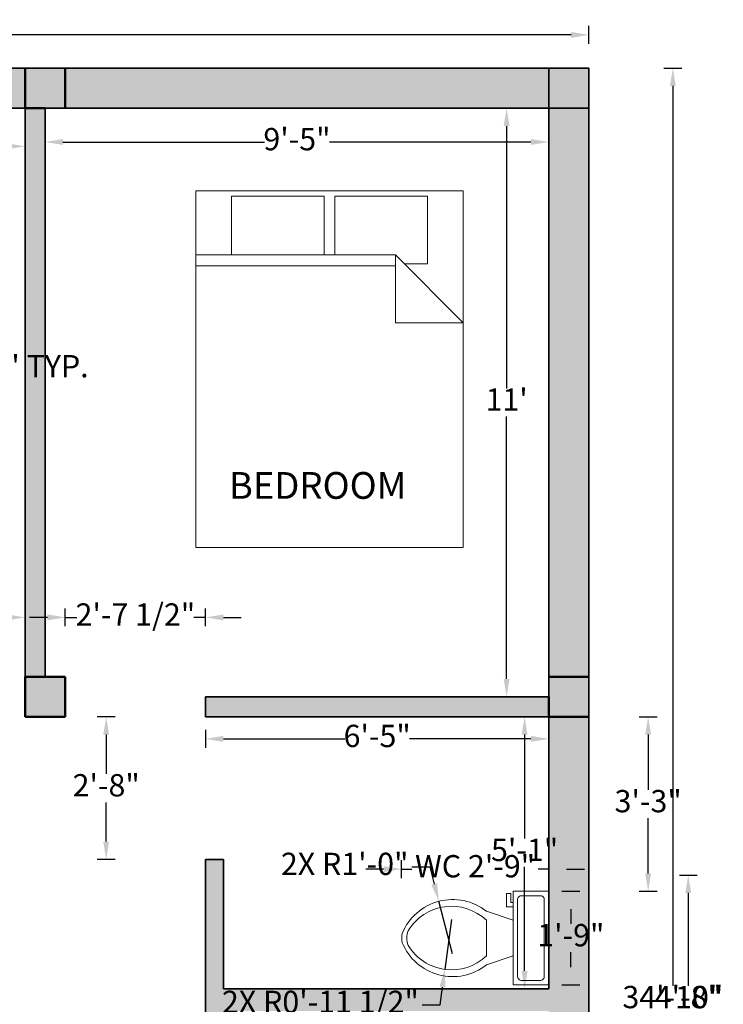
# Model space of a CAD drawing. Units: inches. Extents: x 2244 to 2676, y 593 to 1067.
# Tile 4 of 4: x 2518 to 2676, y 831 to 1052. Entities that reach past the tile are written whole.
import ezdxf

# ---------------------------------------------------------------- set-up
doc = ezdxf.new("R2010")
doc.units = ezdxf.units.IN
for name, color, linetype, lineweight in [('A-ANNO-DIMS', 2, 'Continuous', 18), ('A-AREA-IDEN', 7, 'Continuous', 25), ('A-COLS', 7, 'Continuous', 50), ('A-COLS-PATT', 1, 'Continuous', 13), ('A-FLOR-FIXT', 9, 'Continuous', 18), ('A-FURN', 8, 'Continuous', 18), ('A-WALL', 7, 'Continuous', 35)]:
    doc.layers.add(name, color=color, linetype=linetype, lineweight=lineweight)
doc.layers.add('A-WALL-PATT', color=159, linetype='Continuous', lineweight=13, true_color=0x22346e)
doc.styles.get("Standard").update_dxf_attribs({"font": 'arial.ttf'})
doc.dimstyles.new('ISO-25', dxfattribs={"dimtxt": 5, "dimasz": 4, "dimexe": 2, "dimexo": 2, "dimtad": 0, "dimtih": 1, "dimtoh": 1, "dimlunit": 3, "dimtxsty": 'Standard', "dimcen": 2.5, "dimadec": 0, "dimazin": 0, "dimtfac": 1, "dimtmove": 0, "dimatfit": 3, "dimfxl": 2, "dimfxlon": 1, "dimarcsym": 0})

# ---------------------------------------------------------------- blocks, each defined once
blk = doc.blocks.new('*D6')
at = {"layer": 'A-ANNO-DIMS', "color": 0, "lineweight": -2, "transparency": 16777216}
for p, q in [((2402.7, 1023.38), (2402.7, 1025.38)), ((2519.7, 1023.38), (2519.7, 1025.38)), ((2406.7, 1023.38), (2453.93, 1023.38)), ((2515.7, 1023.38), (2468.47, 1023.38))]:
    blk.add_line(p, q, dxfattribs=at)
at = {"layer": 'A-ANNO-DIMS', "color": 0, "transparency": 16777216}
for points in [[(2406.7, 1024.05), (2406.7, 1022.72), (2402.7, 1023.38)], [(2515.7, 1024.05), (2515.7, 1022.72), (2519.7, 1023.38)]]:
    blk.add_solid(points, dxfattribs=at)
at = {"layer": 'Defpoints', "color": 0, "transparency": 16777216}
for p in [(2402.7, 1023.38), (2402.7, 1022.02), (2519.7, 1022.02)]:
    blk.add_point(p, dxfattribs=at)
at = {"layer": 'A-ANNO-DIMS', "color": 0, "transparency": 16777216, "insert": (2461.2, 1023.38), "char_height": 5, "attachment_point": 5}
blk.add_mtext('9\'-9"', dxfattribs=at)
blk = doc.blocks.new('*D8')
at = {"layer": 'A-ANNO-DIMS', "color": 0, "lineweight": -2, "transparency": 16777216}
for p, q in [((2524.2, 1023.09), (2524.2, 1026.34)), ((2637.2, 1023.09), (2637.2, 1026.34)), ((2528.2, 1024.34), (2573.43, 1024.34)), ((2633.2, 1024.34), (2587.97, 1024.34))]:
    blk.add_line(p, q, dxfattribs=at)
at = {"layer": 'A-ANNO-DIMS', "color": 0, "transparency": 16777216}
for points in [[(2528.2, 1025.01), (2528.2, 1023.68), (2524.2, 1024.34)], [(2633.2, 1025.01), (2633.2, 1023.68), (2637.2, 1024.34)]]:
    blk.add_solid(points, dxfattribs=at)
at = {"layer": 'Defpoints', "color": 0, "transparency": 16777216}
for p in [(2524.2, 1024.34), (2524.2, 1021.09), (2637.2, 1021.09)]:
    blk.add_point(p, dxfattribs=at)
at = {"layer": 'A-ANNO-DIMS', "color": 0, "transparency": 16777216, "insert": (2580.7, 1024.34), "char_height": 5, "attachment_point": 5}
blk.add_mtext('9\'-5"', dxfattribs=at)
blk = doc.blocks.new('*D9')
at = {"layer": 'A-ANNO-DIMS', "color": 0, "lineweight": -2, "transparency": 16777216}
for p, q in [((2626.95, 1031.92), (2629.74, 1031.92)), ((2627.74, 1027.92), (2627.74, 969.06)), ((2627.74, 903.92), (2627.74, 962.79)), ((2626.95, 899.92), (2629.74, 899.92))]:
    blk.add_line(p, q, dxfattribs=at)
at = {"layer": 'A-ANNO-DIMS', "color": 0, "transparency": 16777216}
for points in [[(2627.08, 1027.92), (2628.41, 1027.92), (2627.74, 1031.92)], [(2627.08, 903.92), (2628.41, 903.92), (2627.74, 899.92)]]:
    blk.add_solid(points, dxfattribs=at)
at = {"layer": 'Defpoints', "color": 0, "transparency": 16777216}
for p in [(2624.95, 1031.92), (2624.95, 899.92), (2627.74, 899.92)]:
    blk.add_point(p, dxfattribs=at)
at = {"layer": 'A-ANNO-DIMS', "color": 0, "transparency": 16777216, "insert": (2627.74, 965.92), "char_height": 5, "attachment_point": 5}
blk.add_mtext("11'", dxfattribs=at)
blk = doc.blocks.new('*D11')
at = {"layer": 'A-ANNO-DIMS', "color": 0, "lineweight": -2, "transparency": 16777216}
for p, q in [((2633.78, 895.42), (2629.78, 895.42)), ((2631.78, 891.42), (2631.78, 868.1)), ((2631.78, 838.42), (2631.78, 861.74)), ((2633.78, 834.42), (2629.78, 834.42))]:
    blk.add_line(p, q, dxfattribs=at)
at = {"layer": 'A-ANNO-DIMS', "color": 0, "transparency": 16777216}
for points in [[(2631.11, 891.42), (2632.44, 891.42), (2631.78, 895.42)], [(2631.11, 838.42), (2632.44, 838.42), (2631.78, 834.42)]]:
    blk.add_solid(points, dxfattribs=at)
at = {"layer": 'Defpoints', "color": 0, "transparency": 16777216}
for p in [(2637.2, 895.42), (2631.78, 834.42), (2637.2, 834.42)]:
    blk.add_point(p, dxfattribs=at)
at = {"layer": 'A-ANNO-DIMS', "color": 0, "transparency": 16777216, "insert": (2631.78, 864.92), "char_height": 5, "attachment_point": 5}
blk.add_mtext('5\'-1"', dxfattribs=at)
blk = doc.blocks.new('*D21')
at = {"layer": 'A-ANNO-DIMS', "color": 0, "lineweight": -2, "transparency": 16777216}
for p, q in [((2276.2, 1046.37), (2276.2, 1050.37)), ((2646.2, 1046.37), (2646.2, 1050.37)), ((2280.2, 1048.37), (2450.04, 1048.37)), ((2642.2, 1048.37), (2472.35, 1048.37))]:
    blk.add_line(p, q, dxfattribs=at)
at = {"layer": 'A-ANNO-DIMS', "color": 0, "transparency": 16777216}
for points in [[(2280.2, 1049.03), (2280.2, 1047.7), (2276.2, 1048.37)], [(2642.2, 1049.03), (2642.2, 1047.7), (2646.2, 1048.37)]]:
    blk.add_solid(points, dxfattribs=at)
at = {"layer": 'Defpoints', "color": 0, "transparency": 16777216}
for p in [(2646.2, 1048.37), (2276.2, 1040.92), (2646.2, 1040.92)]:
    blk.add_point(p, dxfattribs=at)
at = {"layer": 'A-ANNO-DIMS', "color": 0, "transparency": 16777216, "insert": (2461.2, 1048.37), "char_height": 5, "attachment_point": 5}
blk.add_mtext('30\'-10"', dxfattribs=at)
blk = doc.blocks.new('*D22')
at = {"layer": 'A-ANNO-DIMS', "color": 0, "lineweight": -2, "transparency": 16777216}
for p, q in [((2663.04, 1040.92), (2667.04, 1040.92)), ((2665.04, 1036.92), (2665.04, 835.1)), ((2665.04, 626.92), (2665.04, 828.74)), ((2663.04, 622.92), (2667.04, 622.92))]:
    blk.add_line(p, q, dxfattribs=at)
at = {"layer": 'A-ANNO-DIMS', "color": 0, "transparency": 16777216}
for points in [[(2664.38, 1036.92), (2665.71, 1036.92), (2665.04, 1040.92)], [(2664.38, 626.92), (2665.71, 626.92), (2665.04, 622.92)]]:
    blk.add_solid(points, dxfattribs=at)
at = {"layer": 'Defpoints', "color": 0, "transparency": 16777216}
for p in [(2646.2, 1040.92), (2646.2, 622.92), (2665.04, 622.92)]:
    blk.add_point(p, dxfattribs=at)
at = {"layer": 'A-ANNO-DIMS', "color": 0, "transparency": 16777216, "insert": (2665.04, 831.92), "char_height": 5, "attachment_point": 5}
blk.add_mtext('34\'-10"', dxfattribs=at)
blk = doc.blocks.new('Bed - Queen')
for p, q in [((0, -80.00003), (0, 0)), ((0, 0), (59.99999, 0)), ((59.99999, 0), (59.99999, -80.00003)), ((7.99999, -1.2), (28.79998, -1.2)), ((7.99999, -14.4), (7.99999, -1.2)), ((28.79998, -1.2), (28.79998, -14.4)), ((31.19999, -1.2), (51.99999, -1.2)), ((31.19999, -14.4), (31.19999, -1.2)), ((51.99999, -1.2), (51.99999, -16.4)), ((0, -14.4), (44.8, -14.4)), ((59.99999, -29.6), (44.8, -14.4)), ((44.8, -14.4), (44.8, -29.6)), ((44.8, -16.8), (0, -16.8)), ((51.99999, -16.4), (46.79936, -16.4)), ((44.8, -29.6), (59.99999, -29.6)), ((59.99999, -80.00003), (0, -80.00003))]:
    blk.add_line(p, q)
blk = doc.blocks.new('Toilet - top')
for p, q in [((9.5, -6), (9.5, -2)), ((-10, -8.5), (-8, -8.5)), ((-10, -9.5), (-10, -8.5)), ((-8, -8.5), (-8, -8)), ((-7, -8), (-7, -9.5)), ((-4, -8), (-6, -14)), ((4, -8), (6, -14)), ((-7, -9.5), (-10, -9.5)), ((4, -14), (-4, -14))]:
    blk.add_line(p, q)
blk.add_lwpolyline([(10.5, -8), (10.5, 0), (-10.5, 0), (-10.5, -8)], close=True)
for points in [[(-9.5, -2), (-9.5, -6)], [(8.5, -1), (-8.5, -1)], [(-8.5, -7), (8.5, -7)]]:
    blk.add_lwpolyline(points)
for centre, radius, start, end in [((-8.62, -1.88), 0.884, 81.8699, 188.1301), ((8.62, -1.88), 0.884, 351.8699, 98.1301), ((-8.62, -6.12), 0.884, 171.8699, 278.1301), ((8.62, -6.12), 0.884, 261.8699, 8.1301), ((3.52, -21.58), 12.17, 141.4691, 247.9714), ((4.2, -21.82), 11.33, 136.3677, 238.9468), ((-3.52, -21.58), 12.17, 292.0284, 38.5307), ((-4.2, -21.82), 11.33, 301.053, 43.6321), ((0, -27.88), 4, 245.7318, 294.2682), ((0, -29), 4, 254.8605, 285.1395)]:
    blk.add_arc(centre, radius, start, end)
blk = doc.blocks.new('*D29')
at = {"layer": 'A-ANNO-DIMS', "color": 0, "lineweight": -2, "transparency": 16777216}
for p, q in [((2560.2, 892.48), (2560.2, 888.48)), ((2637.2, 892.48), (2637.2, 888.48)), ((2564.2, 890.48), (2591.41, 890.48)), ((2633.2, 890.48), (2605.98, 890.48))]:
    blk.add_line(p, q, dxfattribs=at)
at = {"layer": 'A-ANNO-DIMS', "color": 0, "transparency": 16777216}
for points in [[(2564.2, 891.15), (2564.2, 889.81), (2560.2, 890.48)], [(2633.2, 891.15), (2633.2, 889.81), (2637.2, 890.48)]]:
    blk.add_solid(points, dxfattribs=at)
at = {"layer": 'Defpoints', "color": 0, "transparency": 16777216}
for p in [(2560.2, 895.42), (2637.2, 895.42), (2637.2, 890.48)]:
    blk.add_point(p, dxfattribs=at)
at = {"layer": 'A-ANNO-DIMS', "color": 0, "transparency": 16777216, "insert": (2598.7, 890.48), "char_height": 5, "attachment_point": 5}
blk.add_mtext('6\'-5"', dxfattribs=at)
blk = doc.blocks.new('*D30')
at = {"layer": 'A-ANNO-DIMS', "color": 0, "lineweight": -2, "transparency": 16777216}
for p, q in [((2497.1, 1013.41), (2501.1, 1013.41)), ((2499.1, 1009.41), (2499.1, 976.77)), ((2499.1, 937.41), (2499.1, 970.04)), ((2497.1, 933.41), (2501.1, 933.41))]:
    blk.add_line(p, q, dxfattribs=at)
at = {"layer": 'A-ANNO-DIMS', "color": 0, "transparency": 16777216}
for points in [[(2498.44, 1009.41), (2499.77, 1009.41), (2499.1, 1013.41)], [(2498.44, 937.41), (2499.77, 937.41), (2499.1, 933.41)]]:
    blk.add_solid(points, dxfattribs=at)
at = {"layer": 'Defpoints', "color": 0, "transparency": 16777216}
for p in [(2487.1, 1013.41), (2499.1, 1013.41), (2487.1, 933.41)]:
    blk.add_point(p, dxfattribs=at)
at = {"layer": 'A-ANNO-DIMS', "color": 0, "transparency": 16777216, "insert": (2499.1, 973.41), "char_height": 5, "attachment_point": 5}
blk.add_mtext('QUEEN BED 6\'-8" TYP.', dxfattribs=at)
blk = doc.blocks.new('*D34')
at = {"layer": 'A-ANNO-DIMS', "color": 0, "lineweight": -2, "transparency": 16777216}
for p, q in [((2600.15, 861.26), (2596.15, 861.26)), ((2604.15, 859.26), (2604.15, 863.26)), ((2604.15, 861.26), (2606.51, 861.26)), ((2637.2, 861.26), (2634.84, 861.26)), ((2637.2, 859.26), (2637.2, 863.26)), ((2641.2, 861.26), (2645.2, 861.26))]:
    blk.add_line(p, q, dxfattribs=at)
at = {"layer": 'A-ANNO-DIMS', "color": 0, "transparency": 16777216}
for points in [[(2600.15, 861.92), (2600.15, 860.59), (2604.15, 861.26)], [(2641.2, 861.92), (2641.2, 860.59), (2637.2, 861.26)]]:
    blk.add_solid(points, dxfattribs=at)
at = {"layer": 'Defpoints', "color": 0, "transparency": 16777216}
for p in [(2637.2, 861.26), (2604.15, 856.3), (2637.2, 856.3)]:
    blk.add_point(p, dxfattribs=at)
at = {"layer": 'A-ANNO-DIMS', "color": 0, "transparency": 16777216, "insert": (2620.67, 861.26), "char_height": 5, "attachment_point": 5}
blk.add_mtext('WC 2\'-9"', dxfattribs=at)
blk = doc.blocks.new('*D35')
at = {"layer": 'A-ANNO-DIMS', "color": 0, "lineweight": -2, "transparency": 16777216}
for p, q in [((2640.15, 856.3), (2644.15, 856.3)), ((2642.15, 852.3), (2642.15, 848.98)), ((2642.15, 839.3), (2642.15, 842.62)), ((2640.15, 835.3), (2644.15, 835.3))]:
    blk.add_line(p, q, dxfattribs=at)
at = {"layer": 'A-ANNO-DIMS', "color": 0, "transparency": 16777216}
for points in [[(2641.49, 852.3), (2642.82, 852.3), (2642.15, 856.3)], [(2641.49, 839.3), (2642.82, 839.3), (2642.15, 835.3)]]:
    blk.add_solid(points, dxfattribs=at)
at = {"layer": 'Defpoints', "color": 0, "transparency": 16777216}
for p in [(2637.2, 856.3), (2637.2, 835.3), (2642.15, 835.3)]:
    blk.add_point(p, dxfattribs=at)
at = {"layer": 'A-ANNO-DIMS', "color": 0, "transparency": 16777216, "insert": (2642.15, 845.8), "char_height": 5, "attachment_point": 5}
blk.add_mtext('1\'-9"', dxfattribs=at)
blk = doc.blocks.new('*D42')
at = {"layer": 'A-ANNO-DIMS', "color": 0, "lineweight": -2, "transparency": 16777216}
for p, q in [((2666.5, 859.92), (2670.5, 859.92)), ((2668.5, 855.92), (2668.5, 835.1)), ((2668.5, 807.92), (2668.5, 828.74)), ((2666.5, 803.92), (2670.5, 803.92))]:
    blk.add_line(p, q, dxfattribs=at)
at = {"layer": 'A-ANNO-DIMS', "color": 0, "transparency": 16777216}
for points in [[(2667.83, 855.92), (2669.16, 855.92), (2668.5, 859.92)], [(2667.83, 807.92), (2669.16, 807.92), (2668.5, 803.92)]]:
    blk.add_solid(points, dxfattribs=at)
at = {"layer": 'Defpoints', "color": 0, "transparency": 16777216}
for p in [(2359.7, 859.92), (2668.5, 859.92), (2359.7, 803.92)]:
    blk.add_point(p, dxfattribs=at)
at = {"layer": 'A-ANNO-DIMS', "color": 0, "transparency": 16777216, "insert": (2668.5, 831.92), "char_height": 5, "attachment_point": 5}
blk.add_mtext('4\'-8"', dxfattribs=at)
blk = doc.blocks.new('*D44')
at = {"layer": 'A-ANNO-DIMS', "color": 0, "lineweight": -2, "transparency": 16777216}
for p, q in [((2483.7, 915.72), (2483.7, 919.72)), ((2519.7, 915.72), (2519.7, 919.72)), ((2487.7, 917.72), (2494.43, 917.72)), ((2515.7, 917.72), (2508.97, 917.72))]:
    blk.add_line(p, q, dxfattribs=at)
at = {"layer": 'A-ANNO-DIMS', "color": 0, "transparency": 16777216}
for points in [[(2487.7, 918.39), (2487.7, 917.05), (2483.7, 917.72)], [(2515.7, 918.39), (2515.7, 917.05), (2519.7, 917.72)]]:
    blk.add_solid(points, dxfattribs=at)
at = {"layer": 'Defpoints', "color": 0, "transparency": 16777216}
for p in [(2519.7, 917.72), (2483.7, 895.42), (2519.7, 895.42)]:
    blk.add_point(p, dxfattribs=at)
at = {"layer": 'A-ANNO-DIMS', "color": 0, "transparency": 16777216, "insert": (2501.7, 917.72), "char_height": 5, "attachment_point": 5}
blk.add_mtext('3\'-0"', dxfattribs=at)
blk = doc.blocks.new('*D45')
at = {"layer": 'A-ANNO-DIMS', "color": 0, "lineweight": -2, "transparency": 16777216}
for p, q in [((2528.7, 915.72), (2528.7, 919.72)), ((2560.2, 915.72), (2560.2, 919.72)), ((2524.7, 917.72), (2520.7, 917.72)), ((2528.7, 917.72), (2531.31, 917.72)), ((2560.2, 917.72), (2557.59, 917.72)), ((2564.2, 917.72), (2568.2, 917.72))]:
    blk.add_line(p, q, dxfattribs=at)
at = {"layer": 'A-ANNO-DIMS', "color": 0, "transparency": 16777216}
for points in [[(2524.7, 918.39), (2524.7, 917.05), (2528.7, 917.72)], [(2564.2, 918.39), (2564.2, 917.05), (2560.2, 917.72)]]:
    blk.add_solid(points, dxfattribs=at)
at = {"layer": 'Defpoints', "color": 0, "transparency": 16777216}
for p in [(2560.2, 917.72), (2528.7, 895.42), (2560.2, 895.42)]:
    blk.add_point(p, dxfattribs=at)
at = {"layer": 'A-ANNO-DIMS', "color": 0, "transparency": 16777216, "insert": (2544.45, 917.72), "char_height": 5, "attachment_point": 5}
blk.add_mtext('2\'-7 1/2"', dxfattribs=at)
blk = doc.blocks.new('*D46')
at = {"layer": 'A-ANNO-DIMS', "color": 0, "lineweight": -2, "transparency": 16777216}
for p, q in [((2539.9, 895.42), (2535.9, 895.42)), ((2537.9, 891.42), (2537.9, 882.6)), ((2537.9, 867.42), (2537.9, 876.24)), ((2539.9, 863.42), (2535.9, 863.42))]:
    blk.add_line(p, q, dxfattribs=at)
at = {"layer": 'A-ANNO-DIMS', "color": 0, "transparency": 16777216}
for points in [[(2537.23, 891.42), (2538.56, 891.42), (2537.9, 895.42)], [(2537.23, 867.42), (2538.56, 867.42), (2537.9, 863.42)]]:
    blk.add_solid(points, dxfattribs=at)
at = {"layer": 'Defpoints', "color": 0, "transparency": 16777216}
for p in [(2537.9, 895.42), (2560.2, 895.42), (2560.2, 863.42)]:
    blk.add_point(p, dxfattribs=at)
at = {"layer": 'A-ANNO-DIMS', "color": 0, "transparency": 16777216, "insert": (2537.9, 879.42), "char_height": 5, "attachment_point": 5}
blk.add_mtext('2\'-8"', dxfattribs=at)
blk = doc.blocks.new('*D53')
at = {"layer": 'A-ANNO-DIMS', "color": 0, "lineweight": -2, "transparency": 16777216}
for p, q in [((2657.5, 895.42), (2661.5, 895.42)), ((2659.5, 891.42), (2659.5, 879.04)), ((2659.5, 860.3), (2659.5, 872.68)), ((2657.5, 856.3), (2661.5, 856.3))]:
    blk.add_line(p, q, dxfattribs=at)
at = {"layer": 'A-ANNO-DIMS', "color": 0, "transparency": 16777216}
for points in [[(2658.83, 891.42), (2660.16, 891.42), (2659.5, 895.42)], [(2658.83, 860.3), (2660.16, 860.3), (2659.5, 856.3)]]:
    blk.add_solid(points, dxfattribs=at)
at = {"layer": 'Defpoints', "color": 0, "transparency": 16777216}
for p in [(2637.2, 895.42), (2637.2, 856.3), (2659.5, 856.3)]:
    blk.add_point(p, dxfattribs=at)
at = {"layer": 'A-ANNO-DIMS', "color": 0, "transparency": 16777216, "insert": (2659.5, 875.86), "char_height": 5, "attachment_point": 5}
blk.add_mtext('3\'-3"', dxfattribs=at)
blk = doc.blocks.new('*D58')
at = {"layer": 'A-ANNO-DIMS', "color": 0, "lineweight": -2, "transparency": 16777216}
for p, q in [((2606.49, 861.79), (2610.49, 861.79)), ((2610.49, 861.79), (2611.51, 857.92)), ((2615.62, 842.28), (2612.52, 854.05))]:
    blk.add_line(p, q, dxfattribs=at)
at = {"layer": 'A-ANNO-DIMS', "color": 0, "transparency": 16777216}
blk.add_solid([(2612.15, 858.09), (2610.86, 857.75), (2612.52, 854.05)], dxfattribs=at)
at = {"layer": 'Defpoints', "color": 0, "transparency": 16777216}
for p in [(2612.52, 854.05), (2615.62, 842.28)]:
    blk.add_point(p, dxfattribs=at)
at = {"layer": 'A-ANNO-DIMS', "color": 0, "transparency": 16777216, "insert": (2591.41, 861.79), "char_height": 5, "attachment_point": 5}
blk.add_mtext('2X R1\'-0"', dxfattribs=at)
blk = doc.blocks.new('*D59')
at = {"layer": 'A-ANNO-DIMS', "color": 0, "lineweight": -2, "transparency": 16777216}
for p, q in [((2615.38, 850), (2613.87, 838.77)), ((2612.8, 830.84), (2613.34, 834.81)), ((2608.8, 830.84), (2612.8, 830.84))]:
    blk.add_line(p, q, dxfattribs=at)
at = {"layer": 'A-ANNO-DIMS', "color": 0, "transparency": 16777216}
blk.add_solid([(2612.68, 834.9), (2614, 834.72), (2613.87, 838.77)], dxfattribs=at)
at = {"layer": 'Defpoints', "color": 0, "transparency": 16777216}
for p in [(2615.38, 850), (2613.87, 838.77)]:
    blk.add_point(p, dxfattribs=at)
at = {"layer": 'A-ANNO-DIMS', "color": 0, "transparency": 16777216, "insert": (2585.96, 830.84), "char_height": 5, "attachment_point": 5}
blk.add_mtext('2X R0\'-11 1/2"', dxfattribs=at)

msp = doc.modelspace()

# ---------------------------------------------------------------- hatches: boundary and pattern name
at = {"layer": 'A-COLS-PATT'}
h = msp.add_hatch(color=256, dxfattribs=at)
h.dxf.hatch_style = 1
h.paths.add_polyline_path([(2285.197, 1040.922), (2276.197, 1040.922), (2276.197, 1031.922), (2285.197, 1031.922)])
h.paths.add_polyline_path([(2402.697, 1040.922), (2393.697, 1040.922), (2393.697, 1031.922), (2398.197, 1031.922), (2402.697, 1031.922)])
h.paths.add_polyline_path([(2528.697, 1040.922), (2519.697, 1040.922), (2519.697, 1031.922), (2524.197, 1031.922), (2528.697, 1031.922)])
h.paths.add_polyline_path([(2646.197, 1040.922), (2637.197, 1040.922), (2637.197, 1031.922), (2646.197, 1031.922)])
h.paths.add_polyline_path([(2646.197, 904.422), (2637.197, 904.422), (2637.197, 899.922), (2637.197, 895.422), (2646.197, 895.422)])
h.paths.add_polyline_path([(2528.697, 904.422), (2519.697, 904.422), (2519.697, 895.422), (2524.197, 895.422), (2528.697, 895.422)])
h.paths.add_polyline_path([(2402.697, 899.922), (2402.697, 904.422), (2393.697, 904.422), (2393.697, 895.422), (2402.697, 895.422)])
h.paths.add_polyline_path([(2285.197, 899.922), (2285.197, 904.422), (2276.197, 904.422), (2276.197, 895.422), (2285.197, 895.422)])
h.paths.add_polyline_path([(2285.197, 768.422), (2276.197, 768.422), (2276.197, 759.422), (2285.197, 759.422), (2285.197, 763.922)])
h.paths.add_polyline_path([(2285.197, 631.922), (2276.197, 631.922), (2276.197, 622.922), (2285.197, 622.922)])
h.paths.add_polyline_path([(2402.697, 631.922), (2398.197, 631.922), (2393.697, 631.922), (2393.697, 622.922), (2402.697, 622.922)])
h.paths.add_polyline_path([(2402.697, 763.922), (2402.697, 768.422), (2398.197, 768.422), (2393.697, 768.422), (2393.697, 759.422), (2402.697, 759.422)])
h.paths.add_polyline_path([(2528.697, 768.422), (2524.197, 768.422), (2519.697, 768.422), (2519.697, 759.422), (2528.697, 759.422)])
h.paths.add_polyline_path([(2528.697, 631.922), (2524.197, 631.922), (2519.697, 631.922), (2519.697, 628.922), (2519.697, 622.922), (2528.697, 622.922)])
h.paths.add_polyline_path([(2646.197, 631.922), (2637.197, 631.922), (2637.197, 622.922), (2646.197, 622.922)])
h.paths.add_polyline_path([(2646.197, 768.422), (2637.197, 768.422), (2637.197, 763.922), (2637.197, 759.422), (2646.197, 759.422)])
at = {"layer": 'A-WALL-PATT'}
h = msp.add_hatch(color=256, dxfattribs=at)
h.dxf.hatch_style = 1
h.paths.add_polyline_path([(2637.197, 1040.922), (2528.697, 1040.922), (2528.697, 1031.922), (2637.197, 1031.922)])
h.paths.add_polyline_path([(2519.697, 1040.922), (2402.697, 1040.922), (2402.697, 1031.922), (2519.697, 1031.922)])
h.paths.add_polyline_path([(2393.697, 1040.922), (2285.197, 1040.922), (2285.197, 1031.922), (2393.697, 1031.922)])
h.paths.add_polyline_path([(2285.197, 1031.922), (2276.197, 1031.922), (2276.197, 904.422), (2285.197, 904.422)])
h.paths.add_polyline_path([(2402.697, 1031.922), (2398.197, 1031.922), (2398.197, 904.422), (2402.697, 904.422)])
h.paths.add_polyline_path([(2483.697, 899.922), (2402.697, 899.922), (2402.697, 895.422), (2483.697, 895.422)])
h.paths.add_polyline_path([(2524.197, 1031.922), (2519.697, 1031.922), (2519.697, 904.422), (2524.197, 904.422)])
h.paths.add_polyline_path([(2637.197, 899.922), (2560.197, 899.922), (2560.197, 895.422), (2637.197, 895.422)])
h.paths.add_polyline_path([(2646.197, 1031.922), (2637.197, 1031.922), (2637.197, 904.422), (2646.197, 904.422)])
h.paths.add_polyline_path([(2646.197, 895.422), (2637.197, 895.422), (2637.197, 834.422), (2564.197, 834.422), (2564.197, 863.422), (2560.197, 863.422), (2560.197, 800.422), (2564.197, 800.422), (2564.197, 829.422), (2637.197, 829.422), (2637.197, 768.422), (2646.197, 768.422)])
h.paths.add_polyline_path([(2646.197, 759.422), (2637.197, 759.422), (2637.197, 631.922), (2646.197, 631.922)])
h.paths.add_polyline_path([(2637.197, 768.422), (2560.197, 768.422), (2560.197, 763.922), (2637.197, 763.922)])
h.paths.add_polyline_path([(2637.197, 631.922), (2528.697, 631.922), (2528.697, 622.922), (2637.197, 622.922)])
h.paths.add_polyline_path([(2524.197, 759.422), (2519.697, 759.422), (2519.697, 631.922), (2524.197, 631.922)])
h.paths.add_polyline_path([(2402.697, 759.422), (2398.197, 759.422), (2398.197, 631.922), (2402.697, 631.922)])
h.paths.add_polyline_path([(2476.697, 768.422), (2402.697, 768.422), (2402.697, 763.922), (2476.697, 763.922)])
h.paths.add_polyline_path([(2459.697, 631.922), (2402.697, 631.922), (2402.697, 622.922), (2459.697, 622.922), (2459.697, 628.922)])
h.paths.add_polyline_path([(2393.697, 631.922), (2285.197, 631.922), (2285.197, 622.922), (2393.697, 622.922)])
h.paths.add_polyline_path([(2285.197, 759.422), (2276.197, 759.422), (2276.197, 631.922), (2285.197, 631.922)])
h.paths.add_polyline_path([(2359.697, 803.922), (2355.197, 803.922), (2355.197, 768.422), (2285.197, 768.422), (2285.197, 763.922), (2359.697, 763.922)])
h.paths.add_polyline_path([(2359.697, 899.922), (2285.197, 899.922), (2285.197, 895.422), (2355.197, 895.422), (2355.197, 859.922), (2359.697, 859.922)])
h.paths.add_polyline_path([(2285.197, 895.422), (2276.197, 895.422), (2276.197, 768.422), (2285.197, 768.422)])

# ---------------------------------------------------------------- linework, layer by layer
at = {"layer": 'A-COLS'}
for p, q in [((2519.697, 1031.922), (2519.697, 1040.922)), ((2528.697, 1031.922), (2528.697, 1040.922)), ((2519.697, 1031.922), (2524.197, 1031.922)), ((2519.697, 904.422), (2528.697, 904.422)), ((2519.697, 895.422), (2519.697, 904.422)), ((2528.697, 904.422), (2528.697, 895.422)), ((2637.197, 904.422), (2646.197, 904.422)), ((2637.197, 895.422), (2637.197, 899.922)), ((2524.197, 895.422), (2519.697, 895.422)), ((2528.697, 895.422), (2524.197, 895.422)), ((2637.197, 895.422), (2646.197, 895.422))]:
    msp.add_line(p, q, dxfattribs=at)
at = {"layer": 'A-WALL'}
for p, q in [((2646.197, 1040.922), (2276.197, 1040.922)), ((2637.197, 899.922), (2637.197, 1040.922)), ((2646.197, 622.922), (2646.197, 1040.922)), ((2519.697, 1031.922), (2402.697, 1031.922)), ((2519.697, 1031.922), (2519.697, 904.422)), ((2646.197, 1031.922), (2524.197, 1031.922)), ((2524.197, 1031.922), (2524.197, 904.422)), ((2637.197, 899.922), (2560.197, 899.922)), ((2560.197, 899.922), (2560.197, 895.422)), ((2637.197, 895.422), (2560.197, 895.422)), ((2637.197, 834.422), (2637.197, 895.422)), ((2564.197, 863.422), (2560.197, 863.422)), ((2560.197, 800.422), (2560.197, 863.422)), ((2564.197, 834.422), (2564.197, 863.422)), ((2637.197, 834.422), (2564.197, 834.422))]:
    msp.add_line(p, q, dxfattribs=at)

# ---------------------------------------------------------------- block references
at = {"layer": 'A-FLOR-FIXT', "rotation": 270}
msp.add_blockref('Toilet - top', (2637.197, 845.801), dxfattribs=at)
at = {"layer": 'A-FURN'}
msp.add_blockref('Bed - Queen', (2557.987, 1013.405), dxfattribs=at)

# ---------------------------------------------------------------- texts
at = {"layer": 'A-AREA-IDEN', "insert": (2565.422, 950.313), "char_height": 6, "attachment_point": 1}
msp.add_mtext_dynamic_manual_height_columns('BEDROOM', width=31.51274, gutter_width=12.5, heights=[0], dxfattribs=at)

# ---------------------------------------------------------------- dimensions: what is measured, and where the dimension line sits
at = {"layer": 'A-ANNO-DIMS'}
for base, p1, p2, override, picture, middle in [((2646.197, 1048.367), (2276.197, 1040.922), (2646.197, 1040.922), {"dimclrd": 0, "dimclre": 0, "dimclrt": 0}, '*D21', (2461.197, 1048.367)), ((2524.197, 1024.343), (2637.197, 1021.085), (2524.197, 1021.085), {"dimclrd": 0, "dimclre": 0, "dimclrt": 0}, '*D8', (2580.697, 1024.343)), ((2402.697, 1023.385), (2519.697, 1022.016), (2402.697, 1022.016), {"dimclrd": 0, "dimclre": 0, "dimclrt": 0}, '*D6', (2461.197, 1023.385)), ((2560.197, 917.722), (2528.697, 895.422), (2560.197, 895.422), {"dimdec": 1, "dimlfac": 1, "dimrnd": 0, "dimzin": 1, "dimdsep": 46, "dimlunit": 4, "dimfrac": 2}, '*D45', (2544.447, 917.722)), ((2637.197, 890.48), (2560.197, 895.422), (2637.197, 895.422), {"dimclrd": 0, "dimclre": 0, "dimclrt": 0}, '*D29', (2598.697, 890.48))]:
    dim = msp.add_linear_dim(base=base, p1=p1, p2=p2, dimstyle='ISO-25', override=override, dxfattribs=at)
    dim.commit()
    dim.dimension.update_dxf_attribs({"geometry": picture, "text_midpoint": middle})
for base, p1, p2, angle, override, picture, middle in [((2665.043, 622.922), (2646.197, 1040.922), (2646.197, 622.922), 90, {"dimclrd": 0, "dimclre": 0, "dimclrt": 0}, '*D22', (2665.043, 831.922)), ((2627.745, 899.922), (2624.949, 1031.922), (2624.949, 899.922), 90, {"dimclrd": 0, "dimclre": 0, "dimclrt": 0}, '*D9', (2627.745, 965.922)), ((2519.697, 917.722), (2483.697, 895.422), (2519.697, 895.422), 0, {"dimdec": 1, "dimlfac": 1, "dimrnd": 0, "dimzin": 1, "dimdsep": 46, "dimlunit": 4, "dimfrac": 2}, '*D44', (2501.697, 917.722)), ((2537.897, 895.422), (2560.197, 863.422), (2560.197, 895.422), 90, {"dimdec": 1, "dimlfac": 1, "dimrnd": 0, "dimzin": 1, "dimdsep": 46, "dimlunit": 4, "dimfrac": 2}, '*D46', (2537.897, 879.422)), ((2631.776, 834.422), (2637.197, 895.422), (2637.197, 834.422), 90, {"dimclrd": 0, "dimclre": 0, "dimclrt": 0}, '*D11', (2631.776, 864.922)), ((2659.497, 856.301), (2637.197, 895.422), (2637.197, 856.301), 270, {"dimdec": 1, "dimlfac": 1, "dimrnd": 0, "dimzin": 1, "dimdsep": 46, "dimlunit": 4, "dimfrac": 2}, '*D53', (2659.497, 875.861)), ((2668.497, 859.922), (2359.697, 803.922), (2359.697, 859.922), 90, {"dimdec": 1, "dimlfac": 1, "dimrnd": 0, "dimzin": 1, "dimdsep": 46, "dimlunit": 4, "dimfrac": 2}, '*D42', (2668.497, 831.922)), ((2642.154, 835.301), (2637.197, 856.301), (2637.197, 835.301), 270, {"dimdec": 1, "dimlfac": 1, "dimrnd": 0, "dimzin": 1, "dimdsep": 46, "dimlunit": 4, "dimfrac": 2}, '*D35', (2642.154, 845.801))]:
    dim = msp.add_linear_dim(base=base, p1=p1, p2=p2, angle=angle, dimstyle='ISO-25', override=override, dxfattribs=at)
    dim.commit()
    dim.dimension.update_dxf_attribs({"geometry": picture, "text_midpoint": middle})
dim = msp.add_linear_dim(base=(2499.102, 1013.405), p1=(2487.102, 933.405), p2=(2487.102, 1013.405), angle=90, text='QUEEN BED <> TYP.', dimstyle='ISO-25', override={"dimdec": 1, "dimlfac": 1, "dimrnd": 0, "dimzin": 1, "dimdsep": 46, "dimlunit": 4, "dimfrac": 2}, dxfattribs=at)
dim.commit()
dim.dimension.update_dxf_attribs({"geometry": '*D30', "text_midpoint": (2499.102, 973.405)})
for center, mpoint, picture, middle in [((2615.616, 842.281), (2612.524, 854.051), '*D58', (2591.414, 861.788)), ((2615.379, 850.001), (2613.87, 838.773), '*D59', (2585.959, 830.844))]:
    dim = msp.add_radius_dim(center=center, mpoint=mpoint, text='2X <>', dimstyle='ISO-25', override={"dimdec": 1, "dimlfac": 1, "dimrnd": 0, "dimzin": 1, "dimdsep": 46, "dimlunit": 4, "dimfrac": 2}, dxfattribs=at)
    dim.commit()
    dim.dimension.update_dxf_attribs({"geometry": picture, "text_midpoint": middle})
dim = msp.add_linear_dim(base=(2637.197, 861.258), p1=(2604.15, 856.301), p2=(2637.197, 856.301), text='WC <>', dimstyle='ISO-25', override={"dimdec": 1, "dimlfac": 1, "dimrnd": 0, "dimzin": 1, "dimdsep": 46, "dimlunit": 4, "dimfrac": 2}, dxfattribs=at)
dim.commit()
dim.dimension.update_dxf_attribs({"geometry": '*D34', "text_midpoint": (2620.673, 861.258)})

doc.saveas('drawing.dxf')
